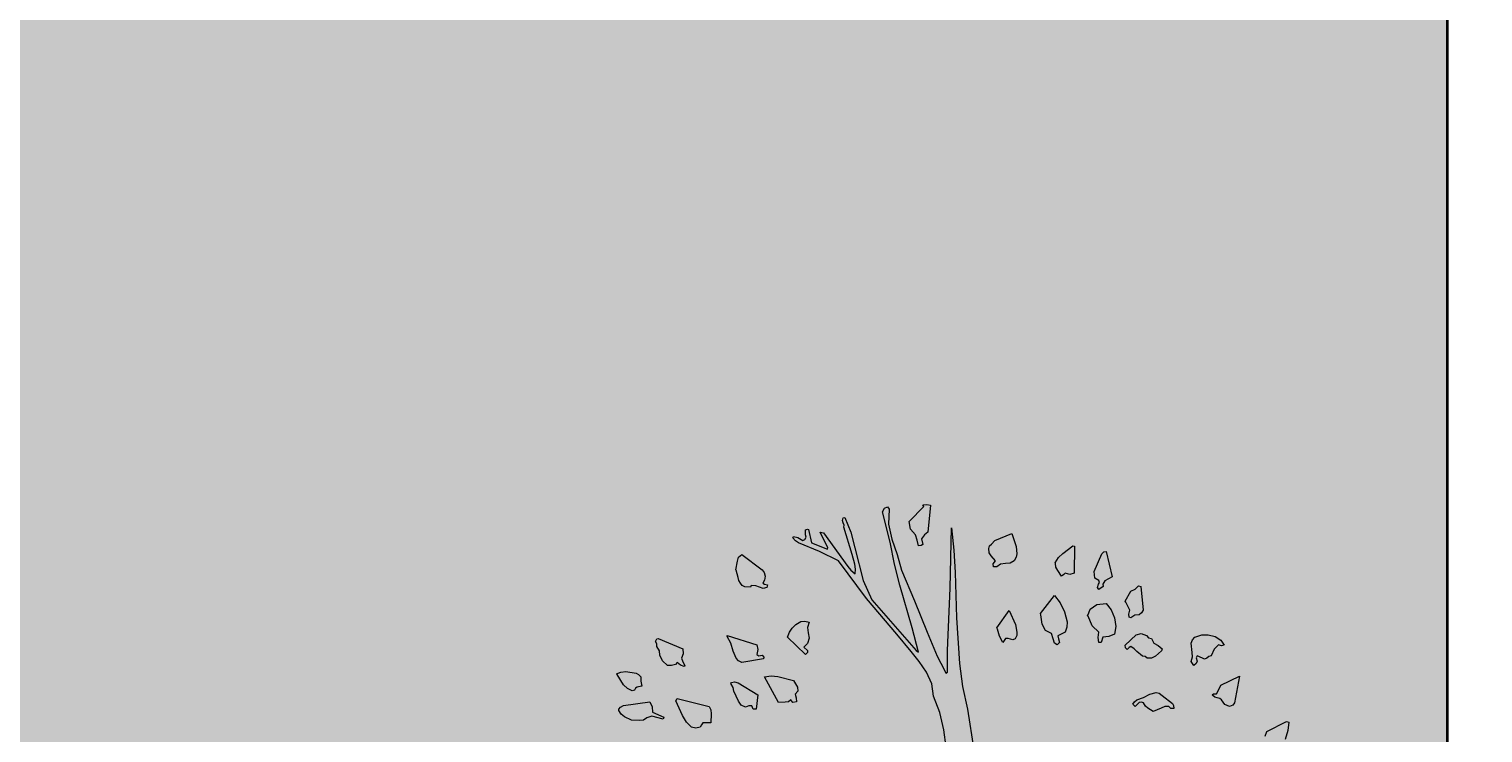
# Model space of a CAD drawing. Units: inches. Extents: x 84 to 1044, y -280 to 906.
# Tile 89 of 105: x 856 to 897, y 426 to 445. Entities that reach past the tile are written whole.
import ezdxf

# ---------------------------------------------------------------- set-up
doc = ezdxf.new("R2010")
doc.units = ezdxf.units.IN
for name, color, linetype, lineweight in [('A-ANNO-DIMS', 2, 'Continuous', 18), ('L-PLNT', 114, 'Continuous', 15), ('WALL', 250, 'Continuous', 35)]:
    doc.layers.add(name, color=color, linetype=linetype, lineweight=lineweight)
doc.layers.add('L-PLNT-PATT', color=9, linetype='Continuous', lineweight=9, true_color=0xafd9aa)
doc.styles.get("Standard").update_dxf_attribs({"font": 'arial.ttf'})
doc.dimstyles.get("Standard").update_dxf_attribs({"dimtxt": 0.18, "dimasz": 0.18, "dimexe": 0.18, "dimexo": 0.0625, "dimgap": 0.09, "dimtad": 0, "dimtih": 1, "dimtoh": 1, "dimdec": 4, "dimzin": 0, "dimdsep": 46, "dimtxsty": 'Standard', "dimcen": 0.09, "dimadec": 0, "dimazin": 0, "dimtfac": 1, "dimtdec": 4, "dimtofl": 0, "dimtmove": 0, "dimatfit": 3, "dimfxl": 1, "dimtolj": 1, "dimtzin": 0, "dimarcsym": 0})

# ---------------------------------------------------------------- blocks, each defined once
blk = doc.blocks.new('A$C37E508DF')
for p, q in [((0.6329, 1.5111), (0.6367, 1.5175)), ((0.6367, 1.5175), (0.6423, 1.5201)), ((0.6423, 1.5201), (0.6453, 1.5158)), ((0.6826, 1.493), (0.7096, 1.5209)), ((0.7083, 1.5239), (0.7152, 1.5244)), ((0.7096, 1.5209), (0.7083, 1.5239)), ((0.7152, 1.5244), (0.7225, 1.5231)), ((0.7225, 1.5231), (0.7174, 1.4729)), ((0.5583, 1.4948), (0.5596, 1.4995)), ((0.5596, 1.4905), (0.5583, 1.4948)), ((0.5596, 1.4995), (0.563, 1.5003)), ((0.5613, 1.4862), (0.5596, 1.4905)), ((0.563, 1.5003), (0.5737, 1.4733)), ((0.6475, 1.4545), (0.6329, 1.5111)), ((0.6453, 1.5158), (0.644, 1.4879)), ((0.6852, 1.4785), (0.6826, 1.493)), ((0.4657, 1.4622), (0.4669, 1.4652)), ((0.4708, 1.4566), (0.4657, 1.4622)), ((0.4669, 1.4652), (0.4755, 1.463)), ((0.4755, 1.463), (0.4845, 1.4575)), ((0.4884, 1.4596), (0.4905, 1.4635)), ((0.4897, 1.4772), (0.4935, 1.4789)), ((0.4897, 1.4678), (0.4897, 1.4772)), ((0.4905, 1.4635), (0.4897, 1.4678)), ((0.4935, 1.4789), (0.4952, 1.478)), ((0.4952, 1.478), (0.5004, 1.4532)), ((0.5313, 1.4437), (0.5167, 1.4729)), ((0.5167, 1.4729), (0.5231, 1.4716)), ((0.5231, 1.4716), (0.5686, 1.409)), ((0.5608, 1.4823), (0.5613, 1.4862)), ((0.5767, 1.4317), (0.5608, 1.4823)), ((0.5737, 1.4733), (0.5814, 1.4437)), ((0.644, 1.4879), (0.6505, 1.46)), ((0.6946, 1.4682), (0.6852, 1.4785)), ((0.6976, 1.4579), (0.6946, 1.4682)), ((0.7109, 1.4682), (0.7053, 1.4609)), ((0.7174, 1.4729), (0.7109, 1.4682)), ((0.7589, 1.3691), (0.7615, 1.481)), ((0.7615, 1.481), (0.7658, 1.4395)), ((0.8421, 1.4575), (0.8739, 1.4703)), ((0.8739, 1.4703), (0.882, 1.4463)), ((0.4764, 1.4532), (0.4708, 1.4566)), ((0.5154, 1.4373), (0.4764, 1.4532)), ((0.4845, 1.4575), (0.4884, 1.4596)), ((0.5004, 1.4532), (0.5308, 1.4412)), ((0.551, 1.4197), (0.5154, 1.4373)), ((0.5308, 1.4412), (0.5313, 1.4437)), ((0.5814, 1.4437), (0.5969, 1.3833)), ((0.6552, 1.4137), (0.6475, 1.4545)), ((0.6505, 1.46), (0.6603, 1.4317)), ((0.7002, 1.4476), (0.6976, 1.4579)), ((0.7049, 1.448), (0.7002, 1.4476)), ((0.7083, 1.4502), (0.7049, 1.448)), ((0.7053, 1.4609), (0.7083, 1.4502)), ((0.7658, 1.4395), (0.7684, 1.3979)), ((0.831, 1.4424), (0.8323, 1.4476)), ((0.8318, 1.4343), (0.831, 1.4424)), ((0.8323, 1.4476), (0.8357, 1.451)), ((0.8357, 1.451), (0.8421, 1.4575)), ((0.882, 1.4463), (0.8829, 1.433)), ((0.9686, 1.4334), (0.9875, 1.4476)), ((0.9875, 1.4476), (0.9905, 1.4467)), ((0.9905, 1.4467), (0.9896, 1.3966)), ((1.0411, 1.433), (1.045, 1.4365)), ((1.045, 1.4365), (1.0497, 1.4369)), ((1.0497, 1.4369), (1.0604, 1.3901)), ((0.3598, 1.403), (0.3628, 1.4189)), ((0.3628, 1.4189), (0.3649, 1.4266)), ((0.3649, 1.4266), (0.3709, 1.4317)), ((0.3709, 1.4317), (0.4086, 1.403)), ((0.6029, 1.3494), (0.551, 1.4197)), ((0.5686, 1.409), (0.5741, 1.4021)), ((0.5814, 1.4133), (0.5767, 1.4317)), ((0.5827, 1.4043), (0.5814, 1.4133)), ((0.6655, 1.3743), (0.6552, 1.4137)), ((0.6603, 1.4317), (0.668, 1.4021)), ((0.8353, 1.4292), (0.8318, 1.4343)), ((0.8434, 1.4197), (0.8353, 1.4292)), ((0.8391, 1.4141), (0.8434, 1.4197)), ((0.8395, 1.4086), (0.8391, 1.4141)), ((0.846, 1.4086), (0.8395, 1.4086)), ((0.8528, 1.4137), (0.846, 1.4086)), ((0.8619, 1.4146), (0.8528, 1.4137)), ((0.8709, 1.4154), (0.8619, 1.4146)), ((0.8781, 1.4197), (0.8709, 1.4154)), ((0.8816, 1.4262), (0.8781, 1.4197)), ((0.8829, 1.433), (0.8816, 1.4262)), ((0.9545, 1.4159), (0.9605, 1.4257)), ((0.9549, 1.4146), (0.9545, 1.4159)), ((0.9558, 1.4077), (0.9549, 1.4146)), ((0.9605, 1.4257), (0.9686, 1.4334)), ((1.0269, 1.3996), (1.0411, 1.433)), ((0.3602, 1.4021), (0.3598, 1.403)), ((0.364, 1.3888), (0.3602, 1.4021)), ((0.3657, 1.3828), (0.364, 1.3888)), ((0.3683, 1.3781), (0.3657, 1.3828)), ((0.4086, 1.403), (0.4125, 1.3979)), ((0.4134, 1.3837), (0.4099, 1.3781)), ((0.4125, 1.3979), (0.4142, 1.391)), ((0.4142, 1.391), (0.4134, 1.3837)), ((0.5741, 1.4021), (0.5823, 1.3953)), ((0.5823, 1.3953), (0.5827, 1.4043)), ((0.5969, 1.3833), (0.6132, 1.3472)), ((0.668, 1.4021), (0.6925, 1.3455)), ((0.7684, 1.3979), (0.771, 1.3134)), ((0.9592, 1.4017), (0.9558, 1.4077)), ((0.966, 1.3914), (0.9592, 1.4017)), ((0.9703, 1.3944), (0.966, 1.3914)), ((0.9733, 1.3966), (0.9703, 1.3944)), ((0.9819, 1.3944), (0.9733, 1.3966)), ((0.9896, 1.3966), (0.9819, 1.3944)), ((1.0282, 1.3876), (1.0269, 1.3996)), ((1.0359, 1.3833), (1.0282, 1.3876)), ((1.0368, 1.3794), (1.0359, 1.3833)), ((1.0471, 1.3824), (1.0432, 1.3764)), ((1.0604, 1.3901), (1.0471, 1.3824)), ((0.3718, 1.3738), (0.3683, 1.3781)), ((0.3765, 1.3713), (0.3718, 1.3738)), ((0.3872, 1.3708), (0.3765, 1.3713)), ((0.3885, 1.3738), (0.3872, 1.3708)), ((0.3971, 1.3734), (0.3885, 1.3738)), ((0.4039, 1.3704), (0.3971, 1.3734)), ((0.4108, 1.3683), (0.4039, 1.3704)), ((0.4099, 1.3781), (0.4134, 1.376)), ((0.4176, 1.37), (0.4108, 1.3683)), ((0.4134, 1.376), (0.4189, 1.3751)), ((0.4189, 1.3751), (0.4176, 1.37)), ((0.6882, 1.2949), (0.6655, 1.3743)), ((0.7538, 1.2529), (0.7589, 1.3691)), ((0.9274, 1.3215), (0.9532, 1.3554)), ((0.9532, 1.3554), (0.9635, 1.3413)), ((1.0334, 1.37), (1.0351, 1.376)), ((1.0359, 1.3661), (1.0334, 1.37)), ((1.0351, 1.376), (1.0368, 1.3794)), ((1.0441, 1.3717), (1.0359, 1.3661)), ((1.0432, 1.3764), (1.0441, 1.3717)), ((1.0848, 1.3443), (1.0955, 1.3631)), ((1.0955, 1.3631), (1.1033, 1.367)), ((1.1033, 1.367), (1.1097, 1.373)), ((1.1097, 1.373), (1.114, 1.3717)), ((1.114, 1.3717), (1.1183, 1.328)), ((0.6595, 1.2829), (0.6029, 1.3494)), ((0.6132, 1.3472), (0.6959, 1.2529)), ((0.6925, 1.3455), (0.7161, 1.2868)), ((0.846, 1.2949), (0.8687, 1.3271)), ((0.8687, 1.3271), (0.8803, 1.3014)), ((0.9635, 1.3413), (0.9721, 1.325)), ((1.0171, 1.3232), (1.0197, 1.3297)), ((1.0197, 1.3297), (1.0321, 1.3387)), ((1.0321, 1.3387), (1.0497, 1.3404)), ((1.0497, 1.3404), (1.0587, 1.3284)), ((1.0587, 1.3284), (1.0651, 1.3134)), ((1.0861, 1.343), (1.0848, 1.3443)), ((1.0938, 1.328), (1.0861, 1.343)), ((1.0917, 1.3207), (1.0938, 1.328)), ((1.1183, 1.328), (1.1153, 1.3228)), ((0.4648, 1.2945), (0.4717, 1.3009)), ((0.4717, 1.3009), (0.4807, 1.3065)), ((0.4807, 1.3065), (0.4884, 1.3074)), ((0.4884, 1.3074), (0.4965, 1.3057)), ((0.4965, 1.3057), (0.4935, 1.2954)), ((0.771, 1.3134), (0.7761, 1.2285)), ((0.8803, 1.3014), (0.8833, 1.2872)), ((0.9279, 1.3194), (0.9274, 1.3215)), ((0.9305, 1.3018), (0.9279, 1.3194)), ((0.9365, 1.2902), (0.9305, 1.3018)), ((0.9721, 1.325), (0.9768, 1.3061)), ((0.9768, 1.3061), (0.9763, 1.2962)), ((1.0149, 1.3172), (1.0171, 1.3232)), ((1.0162, 1.3164), (1.0149, 1.3172)), ((1.0231, 1.2988), (1.0162, 1.3164)), ((1.0651, 1.3134), (1.0677, 1.2975)), ((1.0925, 1.3151), (1.0917, 1.3207)), ((1.0955, 1.3138), (1.0925, 1.3151)), ((1.1028, 1.3185), (1.0955, 1.3138)), ((1.111, 1.3194), (1.1028, 1.3185)), ((1.1153, 1.3228), (1.111, 1.3194)), ((0.2101, 1.2696), (0.2127, 1.2744)), ((0.2127, 1.2744), (0.2152, 1.2752)), ((0.2152, 1.2752), (0.2611, 1.2559)), ((0.3439, 1.2804), (0.3992, 1.2636)), ((0.3439, 1.2787), (0.3439, 1.2804)), ((0.3507, 1.2662), (0.3439, 1.2787)), ((0.4562, 1.2774), (0.4597, 1.2868)), ((0.4897, 1.2452), (0.4562, 1.2774)), ((0.4597, 1.2868), (0.4648, 1.2945)), ((0.4935, 1.2954), (0.4948, 1.2855)), ((0.4961, 1.2756), (0.4935, 1.2658)), ((0.4948, 1.2855), (0.4961, 1.2756)), ((0.6865, 1.2508), (0.6595, 1.2829)), ((0.7002, 1.2495), (0.6882, 1.2949)), ((0.7161, 1.2868), (0.7349, 1.2422)), ((0.8473, 1.2924), (0.846, 1.2949)), ((0.8507, 1.2795), (0.8473, 1.2924)), ((0.8567, 1.2679), (0.8507, 1.2795)), ((0.8619, 1.2752), (0.8567, 1.2679)), ((0.867, 1.2752), (0.8619, 1.2752)), ((0.8713, 1.2739), (0.867, 1.2752)), ((0.8756, 1.2726), (0.8713, 1.2739)), ((0.8799, 1.2744), (0.8756, 1.2726)), ((0.8829, 1.2808), (0.8799, 1.2744)), ((0.8833, 1.2872), (0.8829, 1.2808)), ((0.9476, 1.2842), (0.9365, 1.2902)), ((0.951, 1.2748), (0.9476, 1.2842)), ((0.9532, 1.2666), (0.951, 1.2748)), ((0.9733, 1.2868), (0.9596, 1.2799)), ((0.9596, 1.2799), (0.9605, 1.2744)), ((0.9605, 1.2744), (0.9626, 1.2679)), ((0.9763, 1.2962), (0.9733, 1.2868)), ((1.0359, 1.2868), (1.0231, 1.2988)), ((1.0347, 1.2769), (1.0359, 1.2868)), ((1.0359, 1.2679), (1.0347, 1.2769)), ((1.0432, 1.2774), (1.0402, 1.2679)), ((1.0544, 1.2791), (1.0432, 1.2774)), ((1.0647, 1.2829), (1.0544, 1.2791)), ((1.0677, 1.2975), (1.0647, 1.2829)), ((1.0848, 1.2628), (1.1054, 1.2817)), ((1.1054, 1.2817), (1.1148, 1.2842)), ((1.1148, 1.2842), (1.1247, 1.2804)), ((1.1247, 1.2804), (1.1281, 1.2765)), ((1.1281, 1.2765), (1.1341, 1.2752)), ((1.1341, 1.2752), (1.1384, 1.2666)), ((1.2075, 1.2666), (1.21, 1.2726)), ((1.21, 1.2726), (1.2147, 1.2774)), ((1.2147, 1.2774), (1.2276, 1.2817)), ((1.2276, 1.2817), (1.2392, 1.2817)), ((1.2392, 1.2817), (1.2521, 1.2787)), ((1.2521, 1.2787), (1.2632, 1.2722)), ((0.2127, 1.2654), (0.2101, 1.2696)), ((0.2127, 1.2602), (0.2127, 1.2654)), ((0.2174, 1.2521), (0.2127, 1.2602)), ((0.2182, 1.2443), (0.2174, 1.2521)), ((0.262, 1.2465), (0.2586, 1.2388)), ((0.2611, 1.2559), (0.262, 1.2465)), ((0.3546, 1.2516), (0.3507, 1.2662)), ((0.3602, 1.2383), (0.3546, 1.2516)), ((0.3992, 1.2636), (0.4005, 1.2546)), ((0.4005, 1.2546), (0.3992, 1.2452)), ((0.4935, 1.2658), (0.4867, 1.2589)), ((0.4867, 1.2589), (0.4935, 1.2529)), ((0.4931, 1.2491), (0.4897, 1.2452)), ((0.4935, 1.2529), (0.4931, 1.2491)), ((0.7015, 1.2323), (0.6865, 1.2508)), ((0.6959, 1.2529), (0.7002, 1.2495)), ((0.7538, 1.2122), (0.7538, 1.2529)), ((0.9583, 1.2636), (0.9532, 1.2666)), ((0.9626, 1.2679), (0.9583, 1.2636)), ((1.0402, 1.2679), (1.0359, 1.2679)), ((1.0852, 1.2576), (1.0848, 1.2628)), ((1.0883, 1.2546), (1.0852, 1.2576)), ((1.0921, 1.2585), (1.0883, 1.2546)), ((1.0955, 1.2602), (1.0921, 1.2585)), ((1.1015, 1.2559), (1.0955, 1.2602)), ((1.1063, 1.2508), (1.1015, 1.2559)), ((1.117, 1.2422), (1.1063, 1.2508)), ((1.1384, 1.2666), (1.1461, 1.2619)), ((1.1526, 1.2521), (1.141, 1.2422)), ((1.1461, 1.2619), (1.1539, 1.2559)), ((1.1539, 1.2559), (1.1526, 1.2521)), ((1.2096, 1.2491), (1.2075, 1.2666)), ((1.21, 1.2409), (1.2096, 1.2491)), ((1.2503, 1.2551), (1.2448, 1.2431)), ((1.2585, 1.2636), (1.2503, 1.2551)), ((1.2645, 1.2615), (1.2585, 1.2636)), ((1.2632, 1.2722), (1.2692, 1.2628)), ((1.2692, 1.2628), (1.2645, 1.2615)), ((0.2234, 1.2336), (0.2182, 1.2443)), ((0.2328, 1.2251), (0.2234, 1.2336)), ((0.2401, 1.2251), (0.2328, 1.2251)), ((0.2474, 1.2268), (0.2401, 1.2251)), ((0.2504, 1.2306), (0.2474, 1.2268)), ((0.2568, 1.2255), (0.2504, 1.2306)), ((0.2633, 1.2229), (0.2568, 1.2255)), ((0.2586, 1.2388), (0.2611, 1.2319)), ((0.2611, 1.2319), (0.265, 1.2251)), ((0.265, 1.2251), (0.2633, 1.2229)), ((0.3649, 1.2336), (0.3602, 1.2383)), ((0.3709, 1.2306), (0.3649, 1.2336)), ((0.4112, 1.2375), (0.3709, 1.2306)), ((0.3992, 1.2452), (0.4026, 1.2431)), ((0.4026, 1.2431), (0.4086, 1.2443)), ((0.4086, 1.2443), (0.4121, 1.2401)), ((0.4121, 1.2401), (0.4112, 1.2375)), ((0.7148, 1.2126), (0.7015, 1.2323)), ((0.7349, 1.2422), (0.7482, 1.216)), ((0.7761, 1.2285), (0.7821, 1.1856)), ((1.1221, 1.2418), (1.117, 1.2422)), ((1.126, 1.2388), (1.1221, 1.2418)), ((1.1337, 1.2388), (1.126, 1.2388)), ((1.141, 1.2422), (1.1337, 1.2388)), ((1.2079, 1.2323), (1.21, 1.2409)), ((1.2126, 1.2251), (1.2079, 1.2323)), ((1.2169, 1.2285), (1.2126, 1.2251)), ((1.2186, 1.2332), (1.2169, 1.2285)), ((1.2186, 1.2431), (1.2173, 1.2392)), ((1.2173, 1.2392), (1.2186, 1.2332)), ((1.2285, 1.2383), (1.2186, 1.2431)), ((1.2328, 1.2366), (1.2285, 1.2383)), ((1.2371, 1.2388), (1.2328, 1.2366)), ((1.2405, 1.2418), (1.2371, 1.2388)), ((1.2448, 1.2431), (1.2405, 1.2418)), ((0.1376, 1.2092), (0.1458, 1.2126)), ((0.1389, 1.2079), (0.1376, 1.2092)), ((0.1505, 1.189), (0.1389, 1.2079)), ((0.1458, 1.2126), (0.1548, 1.2135)), ((0.1548, 1.2135), (0.1741, 1.2109)), ((0.1741, 1.2109), (0.1784, 1.2083)), ((0.1784, 1.2083), (0.1831, 1.204)), ((0.1831, 1.204), (0.1831, 1.1959)), ((0.1831, 1.1959), (0.1848, 1.1865)), ((0.3507, 1.1916), (0.352, 1.1933)), ((0.355, 1.1839), (0.3507, 1.1916)), ((0.352, 1.1933), (0.3576, 1.1942)), ((0.3576, 1.1942), (0.364, 1.1929)), ((0.364, 1.1929), (0.4005, 1.1702)), ((0.4134, 1.204), (0.4258, 1.2058)), ((0.4391, 1.156), (0.4134, 1.204)), ((0.4258, 1.2058), (0.4382, 1.2045)), ((0.4382, 1.2045), (0.4669, 1.1972)), ((0.4669, 1.1972), (0.4747, 1.1843)), ((0.7246, 1.1908), (0.7148, 1.2126)), ((0.7482, 1.216), (0.7508, 1.2109)), ((0.7508, 1.2109), (0.7538, 1.2122)), ((1.2628, 1.1882), (1.2975, 1.2053)), ((1.2975, 1.2053), (1.2885, 1.1556)), ((0.1582, 1.1822), (0.1505, 1.189)), ((0.1668, 1.1775), (0.1582, 1.1822)), ((0.1711, 1.1792), (0.1668, 1.1775)), ((0.1728, 1.1826), (0.1711, 1.1792)), ((0.1758, 1.1847), (0.1728, 1.1826)), ((0.1788, 1.1852), (0.1758, 1.1847)), ((0.1848, 1.1865), (0.1788, 1.1852)), ((0.3563, 1.177), (0.355, 1.1839)), ((0.3645, 1.1586), (0.3563, 1.177)), ((0.4005, 1.1702), (0.3979, 1.1436)), ((0.4751, 1.177), (0.47, 1.1714)), ((0.47, 1.1714), (0.4721, 1.1646)), ((0.4721, 1.1646), (0.473, 1.1573)), ((0.4747, 1.1843), (0.4751, 1.177)), ((0.7281, 1.168), (0.7246, 1.1908)), ((0.7396, 1.1371), (0.7281, 1.168)), ((0.7821, 1.1856), (0.7911, 1.1436)), ((1.1063, 1.1612), (1.1187, 1.1655)), ((1.1187, 1.1655), (1.1307, 1.1714)), ((1.1307, 1.1714), (1.1423, 1.1744)), ((1.1423, 1.1744), (1.1483, 1.1732)), ((1.1483, 1.1732), (1.1539, 1.1693)), ((1.1539, 1.1693), (1.1727, 1.1543)), ((1.2469, 1.1702), (1.2495, 1.1723)), ((1.2478, 1.1693), (1.2469, 1.1702)), ((1.2516, 1.1659), (1.2478, 1.1693)), ((1.2495, 1.1723), (1.2546, 1.1719)), ((1.2563, 1.1646), (1.2516, 1.1659)), ((1.2546, 1.1719), (1.2589, 1.1792)), ((1.2611, 1.1637), (1.2563, 1.1646)), ((1.2589, 1.1792), (1.2628, 1.1882)), ((0.1419, 1.1436), (0.1449, 1.1474)), ((0.1419, 1.141), (0.1419, 1.1436)), ((0.1462, 1.1342), (0.1419, 1.141)), ((0.1449, 1.1474), (0.1509, 1.1504)), ((0.1509, 1.1504), (0.1994, 1.1573)), ((0.1994, 1.1573), (0.2041, 1.1479)), ((0.2041, 1.1479), (0.2045, 1.138)), ((0.2045, 1.138), (0.226, 1.129)), ((0.2478, 1.1594), (0.2504, 1.1637)), ((0.2607, 1.1316), (0.2478, 1.1594)), ((0.2504, 1.1637), (0.3104, 1.1487)), ((0.3104, 1.1487), (0.3134, 1.1423)), ((0.3134, 1.1423), (0.3139, 1.1346)), ((0.37, 1.1509), (0.3645, 1.1586)), ((0.3778, 1.1474), (0.37, 1.1509)), ((0.3842, 1.15), (0.3778, 1.1474)), ((0.3898, 1.15), (0.3842, 1.15)), ((0.3923, 1.1436), (0.3898, 1.15)), ((0.3979, 1.1436), (0.3923, 1.1436)), ((0.4519, 1.1564), (0.4391, 1.156)), ((0.458, 1.1573), (0.4519, 1.1564)), ((0.4622, 1.1607), (0.458, 1.1573)), ((0.4657, 1.156), (0.4622, 1.1607)), ((0.473, 1.1573), (0.4657, 1.156)), ((0.7469, 1.1054), (0.7396, 1.1371)), ((0.7911, 1.1436), (0.8027, 1.0677)), ((1.099, 1.153), (1.102, 1.1573)), ((1.1033, 1.1487), (1.099, 1.153)), ((1.102, 1.1573), (1.1063, 1.1612)), ((1.111, 1.156), (1.1033, 1.1487)), ((1.1153, 1.1564), (1.111, 1.156)), ((1.1191, 1.1556), (1.1153, 1.1564)), ((1.1226, 1.1492), (1.1191, 1.1556)), ((1.1273, 1.1453), (1.1226, 1.1492)), ((1.1367, 1.1393), (1.1273, 1.1453)), ((1.1517, 1.1453), (1.1367, 1.1393)), ((1.1586, 1.1483), (1.1517, 1.1453)), ((1.1663, 1.1487), (1.1586, 1.1483)), ((1.1697, 1.1449), (1.1663, 1.1487)), ((1.1757, 1.1449), (1.1697, 1.1449)), ((1.1727, 1.1543), (1.1749, 1.1504)), ((1.1749, 1.1504), (1.1757, 1.1449)), ((1.2641, 1.1612), (1.2611, 1.1637)), ((1.2701, 1.1522), (1.2641, 1.1612)), ((1.2791, 1.1487), (1.2701, 1.1522)), ((1.2851, 1.1509), (1.2791, 1.1487)), ((1.2885, 1.1556), (1.2851, 1.1509)), ((0.1522, 1.1294), (0.1462, 1.1342)), ((0.1655, 1.1234), (0.1522, 1.1294)), ((0.181, 1.1226), (0.1655, 1.1234)), ((0.1878, 1.1234), (0.181, 1.1226)), ((0.1938, 1.1273), (0.1878, 1.1234)), ((0.2032, 1.1303), (0.1938, 1.1273)), ((0.2247, 1.1251), (0.2032, 1.1303)), ((0.226, 1.129), (0.2247, 1.1251)), ((0.268, 1.1196), (0.2607, 1.1316)), ((0.277, 1.1101), (0.268, 1.1196)), ((0.2856, 1.108), (0.277, 1.1101)), ((0.2933, 1.1101), (0.2856, 1.108)), ((0.2959, 1.1144), (0.2933, 1.1101)), ((0.2984, 1.1179), (0.2959, 1.1144)), ((0.3066, 1.1179), (0.2984, 1.1179)), ((0.3134, 1.1183), (0.3066, 1.1179)), ((0.3139, 1.1346), (0.3134, 1.1183)), ((1.3485, 1.102), (1.385, 1.1209)), ((1.385, 1.1209), (1.3897, 1.1196)), ((1.3897, 1.1196), (1.3875, 1.1037)), ((0.7512, 1.0728), (0.7469, 1.1054)), ((1.3455, 1.0934), (1.3485, 1.102)), ((1.3875, 1.1037), (1.3828, 1.087))]:
    blk.add_line(p, q)
blk = doc.blocks.new('*D62')
at = {"layer": 'A-ANNO-DIMS', "color": 0, "lineweight": -2, "transparency": 16777216}
for p, q in [((203.179, 709.183), (203.179, 905.9)), ((896.074, 400.183), (896.074, 905.9)), ((203.359, 905.72), (549.232, 905.72)), ((895.894, 905.72), (550.021, 905.72))]:
    blk.add_line(p, q, dxfattribs=at)
at = {"layer": 'A-ANNO-DIMS', "color": 0, "transparency": 16777216}
for points in [[(203.359, 905.75), (203.359, 905.69), (203.179, 905.72)], [(895.894, 905.75), (895.894, 905.69), (896.074, 905.72)]]:
    blk.add_solid(points, dxfattribs=at)
at = {"layer": 'Defpoints', "color": 0, "transparency": 16777216}
for p in [(896.074, 905.72), (203.179, 709.12), (896.074, 400.12)]:
    blk.add_point(p, dxfattribs=at)
at = {"layer": 'A-ANNO-DIMS', "color": 0, "transparency": 16777216, "insert": (549.627, 905.72), "char_height": 0.18, "attachment_point": 5}
blk.add_mtext('\\A1;692.9', dxfattribs=at)
blk = doc.blocks.new('*D63')
at = {"layer": 'A-ANNO-DIMS', "color": 0, "lineweight": -2, "transparency": 16777216}
for p, q in [((833.136, 709.12), (1043.768, 709.12)), ((1043.588, 708.94), (1043.588, 400.302)), ((1043.588, 91.3), (1043.588, 399.938)), ((896.136, 91.12), (1043.768, 91.12))]:
    blk.add_line(p, q, dxfattribs=at)
at = {"layer": 'A-ANNO-DIMS', "color": 0, "transparency": 16777216}
for points in [[(1043.558, 708.94), (1043.618, 708.94), (1043.588, 709.12)], [(1043.558, 91.3), (1043.618, 91.3), (1043.588, 91.12)]]:
    blk.add_solid(points, dxfattribs=at)
at = {"layer": 'Defpoints', "color": 0, "transparency": 16777216}
for p in [(833.074, 709.12), (1043.588, 709.12), (896.074, 91.12)]:
    blk.add_point(p, dxfattribs=at)
at = {"layer": 'A-ANNO-DIMS', "color": 0, "transparency": 16777216, "insert": (1043.588, 400.12), "char_height": 0.18, "attachment_point": 5}
blk.add_mtext('\\A1;618', dxfattribs=at)
blk = doc.blocks.new('*D65')
at = {"layer": 'A-ANNO-DIMS', "color": 0, "lineweight": -2, "transparency": 16777216}
for p, q in [((896.074, 400.183), (896.074, 905.9)), ((992.074, 856.183), (992.074, 905.9)), ((896.254, 905.72), (943.855, 905.72)), ((991.894, 905.72), (944.293, 905.72))]:
    blk.add_line(p, q, dxfattribs=at)
at = {"layer": 'A-ANNO-DIMS', "color": 0, "transparency": 16777216}
for points in [[(896.254, 905.75), (896.254, 905.69), (896.074, 905.72)], [(991.894, 905.75), (991.894, 905.69), (992.074, 905.72)]]:
    blk.add_solid(points, dxfattribs=at)
at = {"layer": 'Defpoints', "color": 0, "transparency": 16777216}
for p in [(896.074, 905.72), (992.074, 856.12), (896.074, 400.12)]:
    blk.add_point(p, dxfattribs=at)
at = {"layer": 'A-ANNO-DIMS', "color": 0, "transparency": 16777216, "insert": (944.074, 905.72), "char_height": 0.18, "attachment_point": 5}
blk.add_mtext('\\A1;96', dxfattribs=at)

msp = doc.modelspace()

# ---------------------------------------------------------------- hatches: boundary and pattern name
at = {"layer": 'L-PLNT-PATT', "transparency": 33554597}
h = msp.add_hatch(color=256, dxfattribs=at)
h.dxf.hatch_style = 1
h.paths.add_polyline_path([(896.074, 511.12), (704.074, 511.12), (704.074, 491.62), (704.074, 419.62), (704.074, 400.12), (833.074, 400.12), (896.074, 400.12)])

# ---------------------------------------------------------------- linework, layer by layer
at = {"layer": 'WALL'}
msp.add_line((896.074, 400.12), (896.074, 511.12), dxfattribs=at)

# ---------------------------------------------------------------- block references
at = {"layer": 'L-PLNT', "xscale": 15.19586232982809, "yscale": 15.19586232982809, "zscale": 15.19586232982809}
msp.add_blockref('A$C37E508DF', (870.466, 408.868), dxfattribs=at)

# ---------------------------------------------------------------- dimensions: what is measured, and where the dimension line sits
at = {"layer": 'A-ANNO-DIMS'}
for p1, override, picture, middle in [((203.179, 709.12), {"dimdec": 1, "dimlfac": 1, "dimrnd": 0, "dimzin": 0, "dimdsep": 46, "dimlunit": 2}, '*D62', (549.627, 905.72)), ((992.074, 856.12), {"dimdec": 0, "dimlfac": 1, "dimrnd": 0, "dimzin": 0, "dimdsep": 46, "dimlunit": 2}, '*D65', (944.074, 905.72))]:
    dim = msp.add_linear_dim(base=(896.074, 905.72), p1=p1, p2=(896.074, 400.12), dimstyle='Standard', override=override, dxfattribs=at)
    dim.commit()
    dim.dimension.update_dxf_attribs({"geometry": picture, "text_midpoint": middle})
dim = msp.add_linear_dim(base=(1043.588, 709.12), p1=(896.074, 91.12), p2=(833.074, 709.12), angle=90, dimstyle='Standard', override={"dimdec": 0, "dimlfac": 1, "dimrnd": 0, "dimzin": 0, "dimdsep": 46, "dimlunit": 2}, dxfattribs=at)
dim.commit()
dim.dimension.update_dxf_attribs({"geometry": '*D63', "text_midpoint": (1043.588, 400.12)})

doc.saveas('drawing.dxf')
